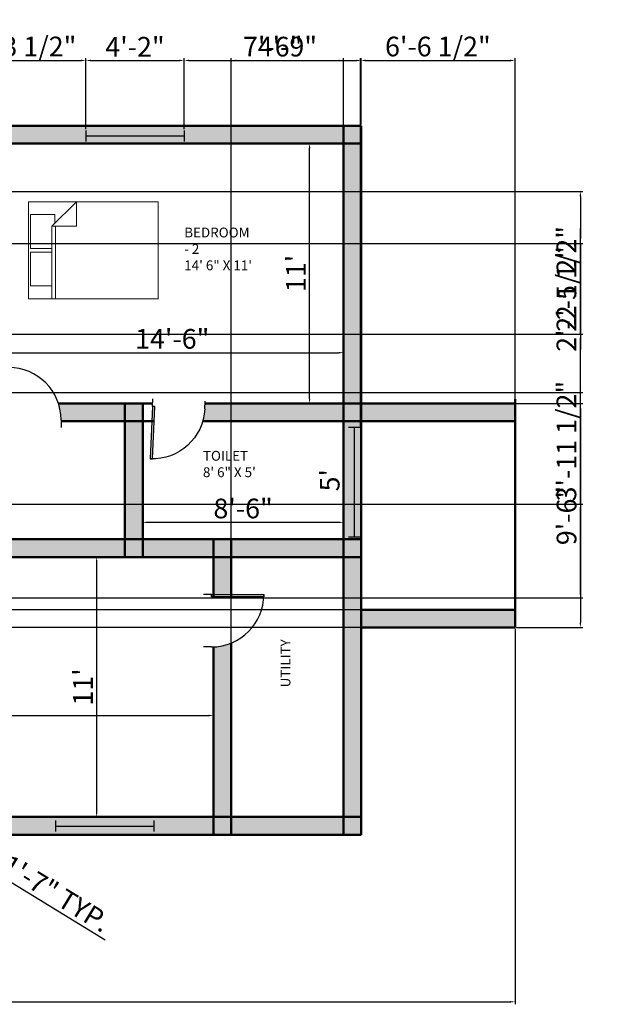
# Model space of a CAD drawing. Units: millimetres. Extents: x 2208 to 3043, y 878 to 1386.
# Tile 4 of 4: x 2749 to 3043, y 886 to 1386. Entities that reach past the tile are written whole.
import ezdxf

# ---------------------------------------------------------------- set-up
doc = ezdxf.new("R2010")
doc.units = ezdxf.units.MM
for name, color, linetype, lineweight in [('A-ANNO-DIMS', 50, 'Continuous', 13), ('A-AREA-IDEN', 90, 'Continuous', 25), ('A-WALL-PATT', 6, 'Continuous', 13), ('doors', 30, 'Continuous', 25), ('furniture', 140, 'Continuous', 18), ('walls', 200, 'Continuous', 50), ('windows', 10, 'Continuous', 25)]:
    doc.layers.add(name, color=color, linetype=linetype, lineweight=lineweight)
doc.styles.get("Standard").update_dxf_attribs({"font": 'arial.ttf'})
doc.dimstyles.new('ISO-25', dxfattribs={"dimtxt": 10, "dimasz": 2.5, "dimexe": 1.25, "dimexo": 0.625, "dimtad": 1, "dimdec": 0, "dimlunit": 3, "dimtxsty": 'Standard', "dimcen": 2.5, "dimadec": 0, "dimazin": 0, "dimtfac": 1, "dimtdec": 0, "dimtmove": 0, "dimatfit": 3, "dimfxl": 1, "dimarcsym": 0})

# ---------------------------------------------------------------- blocks, each defined once
blk = doc.blocks.new('*U2')
for p, q in [((0, 0), (0, -6)), ((40, 0), (40, -6))]:
    blk.add_line(p, q)
blk.add_lwpolyline([(0, 0), (0, 40), (1.75, 40), (1.75, 0)], close=True)
blk.add_arc((0, 0), 40, 0, 90)
blk = doc.blocks.new('*U4')
for p, q in [((0, 4), (0, 0)), ((36, 4), (36, 0)), ((0, 2), (36, 2))]:
    blk.add_line(p, q)
blk = doc.blocks.new('*U5')
for p, q in [((0, 4), (0, 0)), ((36, 4), (36, 0)), ((0, 2), (36, 2))]:
    blk.add_line(p, q)
blk = doc.blocks.new('Bed - Queen')
for p, q in [((0, -80.00003), (0, 0)), ((0, 0), (59.99999, 0)), ((59.99999, 0), (59.99999, -80.00003)), ((7.99999, -1.2), (28.79998, -1.2)), ((7.99999, -14.4), (7.99999, -1.2)), ((28.79998, -1.2), (28.79998, -14.4)), ((31.19999, -1.2), (51.99999, -1.2)), ((31.19999, -14.4), (31.19999, -1.2)), ((51.99999, -1.2), (51.99999, -16.4)), ((0, -14.4), (44.8, -14.4)), ((44.8, -16.8), (0, -16.8)), ((59.99999, -29.6), (44.8, -14.4)), ((44.8, -14.4), (44.8, -29.6)), ((51.99999, -16.4), (46.79936, -16.4)), ((44.8, -29.6), (59.99999, -29.6)), ((59.99999, -80.00003), (0, -80.00003))]:
    blk.add_line(p, q)
blk = doc.blocks.new('*D19')
at = {"layer": 'A-ANNO-DIMS', "color": 0, "lineweight": -2, "transparency": 16777216}
for p, q in [((2739.98, 1223.81), (2739.98, 1215.95)), ((2913.98, 1223.81), (2913.98, 1215.95)), ((2742.48, 1217.2), (2911.48, 1217.2))]:
    blk.add_line(p, q, dxfattribs=at)
at = {"layer": 'A-ANNO-DIMS', "color": 0, "transparency": 16777216}
for points in [[(2742.48, 1217.62), (2742.48, 1216.78), (2739.98, 1217.2)], [(2911.48, 1217.62), (2911.48, 1216.78), (2913.98, 1217.2)]]:
    blk.add_solid(points, dxfattribs=at)
at = {"layer": 'Defpoints', "color": 0, "transparency": 16777216}
for p in [(2739.98, 1224.44), (2913.98, 1224.44), (2913.98, 1217.2)]:
    blk.add_point(p, dxfattribs=at)
at = {"layer": 'A-ANNO-DIMS', "color": 0, "transparency": 16777216, "insert": (2826.98, 1222.93), "char_height": 10, "attachment_point": 5}
blk.add_mtext('14\'-6"', dxfattribs=at)
blk = doc.blocks.new('*D20')
at = {"layer": 'A-ANNO-DIMS', "color": 0, "lineweight": -2, "transparency": 16777216}
for p, q in [((2887.05, 1323.44), (2898, 1323.44)), ((2896.75, 1193.94), (2896.75, 1320.94)), ((2887.05, 1191.44), (2898, 1191.44))]:
    blk.add_line(p, q, dxfattribs=at)
at = {"layer": 'A-ANNO-DIMS', "color": 0, "transparency": 16777216}
for points in [[(2896.33, 1320.94), (2897.16, 1320.94), (2896.75, 1323.44)], [(2896.33, 1193.94), (2897.16, 1193.94), (2896.75, 1191.44)]]:
    blk.add_solid(points, dxfattribs=at)
at = {"layer": 'Defpoints', "color": 0, "transparency": 16777216}
for p in [(2886.43, 1323.44), (2896.75, 1323.44), (2886.43, 1191.44)]:
    blk.add_point(p, dxfattribs=at)
at = {"layer": 'A-ANNO-DIMS', "color": 0, "transparency": 16777216, "insert": (2891.1, 1257.44), "char_height": 10, "attachment_point": 5, "rotation": 90}
blk.add_mtext("11'", dxfattribs=at)
blk = doc.blocks.new('*D27')
at = {"layer": 'A-ANNO-DIMS', "color": 0, "lineweight": -2, "transparency": 16777216}
for p, q in [((2598.98, 1051.4), (2598.98, 1031.71)), ((2847.98, 1051.4), (2847.98, 1031.71)), ((2601.48, 1032.96), (2845.48, 1032.96))]:
    blk.add_line(p, q, dxfattribs=at)
at = {"layer": 'A-ANNO-DIMS', "color": 0, "transparency": 16777216}
for points in [[(2601.48, 1033.38), (2601.48, 1032.54), (2598.98, 1032.96)], [(2845.48, 1033.38), (2845.48, 1032.54), (2847.98, 1032.96)]]:
    blk.add_solid(points, dxfattribs=at)
at = {"layer": 'Defpoints', "color": 0, "transparency": 16777216}
for p in [(2598.98, 1052.02), (2847.98, 1052.02), (2847.98, 1032.96)]:
    blk.add_point(p, dxfattribs=at)
at = {"layer": 'A-ANNO-DIMS', "color": 0, "transparency": 16777216, "insert": (2723.48, 1038.69), "char_height": 10, "attachment_point": 5}
blk.add_mtext('20\'-9"', dxfattribs=at)
blk = doc.blocks.new('*D28')
at = {"layer": 'A-ANNO-DIMS', "color": 0, "lineweight": -2, "transparency": 16777216}
for p, q in [((2764.06, 1113.44), (2789.84, 1113.44)), ((2788.59, 1110.94), (2788.59, 983.94)), ((2764.06, 981.44), (2789.84, 981.44))]:
    blk.add_line(p, q, dxfattribs=at)
at = {"layer": 'A-ANNO-DIMS', "color": 0, "transparency": 16777216}
for points in [[(2788.18, 1110.94), (2789.01, 1110.94), (2788.59, 1113.44)], [(2788.18, 983.94), (2789.01, 983.94), (2788.59, 981.44)]]:
    blk.add_solid(points, dxfattribs=at)
at = {"layer": 'Defpoints', "color": 0, "transparency": 16777216}
for p in [(2763.44, 1113.44), (2763.44, 981.44), (2788.59, 981.44)]:
    blk.add_point(p, dxfattribs=at)
at = {"layer": 'A-ANNO-DIMS', "color": 0, "transparency": 16777216, "insert": (2782.95, 1047.44), "char_height": 10, "attachment_point": 5, "rotation": 90}
blk.add_mtext("11'", dxfattribs=at)
blk = doc.blocks.new('*D29')
at = {"layer": 'A-ANNO-DIMS', "color": 0, "lineweight": -2, "transparency": 16777216}
for p, q in [((2811.98, 1144.04), (2811.98, 1129.82)), ((2913.98, 1144.04), (2913.98, 1129.82)), ((2814.48, 1131.07), (2911.48, 1131.07))]:
    blk.add_line(p, q, dxfattribs=at)
at = {"layer": 'A-ANNO-DIMS', "color": 0, "transparency": 16777216}
for points in [[(2814.48, 1131.48), (2814.48, 1130.65), (2811.98, 1131.07)], [(2911.48, 1131.48), (2911.48, 1130.65), (2913.98, 1131.07)]]:
    blk.add_solid(points, dxfattribs=at)
at = {"layer": 'Defpoints', "color": 0, "transparency": 16777216}
for p in [(2811.98, 1144.67), (2913.98, 1144.67), (2913.98, 1131.07)]:
    blk.add_point(p, dxfattribs=at)
at = {"layer": 'A-ANNO-DIMS', "color": 0, "transparency": 16777216, "insert": (2862.98, 1136.8), "char_height": 10, "attachment_point": 5}
blk.add_mtext('8\'-6"', dxfattribs=at)
blk = doc.blocks.new('*D30')
at = {"layer": 'A-ANNO-DIMS', "color": 0, "lineweight": -2, "transparency": 16777216}
for p, q in [((2900.41, 1182.44), (2915.23, 1182.44)), ((2913.98, 1124.94), (2913.98, 1179.94)), ((2900.41, 1122.44), (2915.23, 1122.44))]:
    blk.add_line(p, q, dxfattribs=at)
at = {"layer": 'A-ANNO-DIMS', "color": 0, "transparency": 16777216}
for points in [[(2913.57, 1179.94), (2914.4, 1179.94), (2913.98, 1182.44)], [(2913.57, 1124.94), (2914.4, 1124.94), (2913.98, 1122.44)]]:
    blk.add_solid(points, dxfattribs=at)
at = {"layer": 'Defpoints', "color": 0, "transparency": 16777216}
for p in [(2899.78, 1182.44), (2913.98, 1182.44), (2899.78, 1122.44)]:
    blk.add_point(p, dxfattribs=at)
at = {"layer": 'A-ANNO-DIMS', "color": 0, "transparency": 16777216, "insert": (2908.27, 1152.44), "char_height": 10, "attachment_point": 5, "rotation": 90}
blk.add_mtext("5'", dxfattribs=at)
blk = doc.blocks.new('*D38')
at = {"layer": 'A-ANNO-DIMS', "color": 0, "lineweight": -2, "transparency": 16777216}
for p, q in [((2680.05, 985.52), (2681.86, 988.48)), ((2683.34, 986.11), (2695.25, 978.83)), ((2696.22, 975.63), (2698.03, 978.59)), ((2697.38, 977.52), (2792.87, 919.11))]:
    blk.add_line(p, q, dxfattribs=at)
at = {"layer": 'A-ANNO-DIMS', "color": 0, "transparency": 16777216}
for points in [[(2683.56, 986.47), (2683.13, 985.76), (2681.21, 987.42)], [(2695.47, 979.18), (2695.03, 978.47), (2697.38, 977.52)]]:
    blk.add_solid(points, dxfattribs=at)
at = {"layer": 'Defpoints', "color": 0, "transparency": 16777216}
for p in [(2679.73, 984.99), (2695.9, 975.1), (2697.38, 977.52)]:
    blk.add_point(p, dxfattribs=at)
at = {"layer": 'A-ANNO-DIMS', "color": 0, "transparency": 16777216, "insert": (2749.21, 952.61), "char_height": 10, "attachment_point": 5, "rotation": 328.5439}
blk.add_mtext('CHAIR 1\'-7" TYP.', dxfattribs=at)
blk = doc.blocks.new('*D46')
at = {"layer": 'A-ANNO-DIMS', "color": 0, "lineweight": -2, "transparency": 16777216}
for p, q in [((3001.16, 1077), (3001.16, 886.32)), ((2343.98, 972.81), (2343.98, 886.32)), ((2346.48, 887.57), (2998.66, 887.57))]:
    blk.add_line(p, q, dxfattribs=at)
at = {"layer": 'A-ANNO-DIMS', "color": 0, "transparency": 16777216}
for points in [[(2346.48, 887.99), (2346.48, 887.16), (2343.98, 887.57)], [(2998.66, 887.99), (2998.66, 887.16), (3001.16, 887.57)]]:
    blk.add_solid(points, dxfattribs=at)
at = {"layer": 'Defpoints', "color": 0, "transparency": 16777216}
for p in [(3001.16, 1077.62), (2343.98, 973.44), (3001.16, 887.57)]:
    blk.add_point(p, dxfattribs=at)
at = {"layer": 'A-ANNO-DIMS', "color": 0, "transparency": 16777216, "insert": (2672.57, 893.3), "char_height": 10, "attachment_point": 5}
blk.add_mtext('54\'-9"', dxfattribs=at)
blk = doc.blocks.new('*D48')
at = {"layer": 'A-ANNO-DIMS', "color": 0, "lineweight": -2, "transparency": 16777216}
for p, q in [((2922.7, 1179.95), (2922.7, 1366.84)), ((2925.2, 1365.59), (2998.66, 1365.59)), ((3001.16, 1192.06), (3001.16, 1366.84))]:
    blk.add_line(p, q, dxfattribs=at)
at = {"layer": 'A-ANNO-DIMS', "color": 0, "transparency": 16777216}
for points in [[(2925.2, 1366), (2925.2, 1365.17), (2922.7, 1365.59)], [(2998.66, 1366), (2998.66, 1365.17), (3001.16, 1365.59)]]:
    blk.add_solid(points, dxfattribs=at)
at = {"layer": 'Defpoints', "color": 0, "transparency": 16777216}
for p in [(3001.16, 1365.59), (3001.16, 1191.44), (2922.7, 1179.32)]:
    blk.add_point(p, dxfattribs=at)
at = {"layer": 'A-ANNO-DIMS', "color": 0, "transparency": 16777216, "insert": (2961.93, 1371.38), "char_height": 10, "attachment_point": 5}
blk.add_mtext('6\'-6 1/2"', dxfattribs=at)
blk = doc.blocks.new('*D49')
at = {"layer": 'A-ANNO-DIMS', "color": 0, "lineweight": -2, "transparency": 16777216}
for p, q in [((3001.79, 1191.44), (3035.56, 1191.44)), ((3034.31, 1188.94), (3034.31, 1080.12)), ((3001.79, 1077.62), (3035.56, 1077.62))]:
    blk.add_line(p, q, dxfattribs=at)
at = {"layer": 'A-ANNO-DIMS', "color": 0, "transparency": 16777216}
for points in [[(3033.9, 1188.94), (3034.73, 1188.94), (3034.31, 1191.44)], [(3033.9, 1080.12), (3034.73, 1080.12), (3034.31, 1077.62)]]:
    blk.add_solid(points, dxfattribs=at)
at = {"layer": 'Defpoints', "color": 0, "transparency": 16777216}
for p in [(3001.16, 1191.44), (3001.16, 1077.62), (3034.31, 1077.62)]:
    blk.add_point(p, dxfattribs=at)
at = {"layer": 'A-ANNO-DIMS', "color": 0, "transparency": 16777216, "insert": (3028.58, 1134.53), "char_height": 10, "attachment_point": 5, "rotation": 90}
blk.add_mtext('9\'-6"', dxfattribs=at)
blk = doc.blocks.new('*D50')
at = {"layer": 'A-ANNO-DIMS', "color": 0, "lineweight": -2, "transparency": 16777216}
for p, q in [((2856.98, 973.06), (2856.98, 1366.84)), ((2859.48, 1365.59), (2911.48, 1365.59)), ((2913.98, 973.06), (2913.98, 1366.84))]:
    blk.add_line(p, q, dxfattribs=at)
at = {"layer": 'A-ANNO-DIMS', "color": 0, "transparency": 16777216}
for points in [[(2859.48, 1366), (2859.48, 1365.17), (2856.98, 1365.59)], [(2911.48, 1366), (2911.48, 1365.17), (2913.98, 1365.59)]]:
    blk.add_solid(points, dxfattribs=at)
at = {"layer": 'Defpoints', "color": 0, "transparency": 16777216}
for p in [(2913.98, 1365.59), (2856.98, 972.44), (2913.98, 972.44)]:
    blk.add_point(p, dxfattribs=at)
at = {"layer": 'A-ANNO-DIMS', "color": 0, "transparency": 16777216, "insert": (2885.48, 1371.32), "char_height": 10, "attachment_point": 5}
blk.add_mtext('4\'-9"', dxfattribs=at)
blk = doc.blocks.new('*D51')
at = {"layer": 'A-ANNO-DIMS', "color": 0, "lineweight": -2, "transparency": 16777216}
for p, q in [((2344.15, 1299.03), (3035.56, 1299.03)), ((3034.31, 1296.53), (3034.31, 1275.14)), ((2344.61, 1272.64), (3035.56, 1272.64)), ((3034.31, 1272.64), (3034.31, 1218.83))]:
    blk.add_line(p, q, dxfattribs=at)
at = {"layer": 'A-ANNO-DIMS', "color": 0, "transparency": 16777216}
for points in [[(3033.9, 1296.53), (3034.73, 1296.53), (3034.31, 1299.03)], [(3033.9, 1275.14), (3034.73, 1275.14), (3034.31, 1272.64)]]:
    blk.add_solid(points, dxfattribs=at)
at = {"layer": 'Defpoints', "color": 0, "transparency": 16777216}
for p in [(2343.52, 1299.03), (2343.98, 1272.64), (3034.31, 1272.64)]:
    blk.add_point(p, dxfattribs=at)
at = {"layer": 'A-ANNO-DIMS', "color": 0, "transparency": 16777216, "insert": (3028.52, 1244.49), "char_height": 10, "attachment_point": 5, "rotation": 90}
blk.add_mtext('2\'-2 1/2"', dxfattribs=at)
blk = doc.blocks.new('*D59')
at = {"layer": 'A-ANNO-DIMS', "color": 0, "lineweight": -2, "transparency": 16777216}
for p, q in [((2719.8, 1331.57), (2719.8, 1366.84)), ((2722.3, 1365.59), (2780.58, 1365.59)), ((2783.08, 1330.66), (2783.08, 1366.84))]:
    blk.add_line(p, q, dxfattribs=at)
at = {"layer": 'A-ANNO-DIMS', "color": 0, "transparency": 16777216}
for points in [[(2722.3, 1366), (2722.3, 1365.17), (2719.8, 1365.59)], [(2780.58, 1366), (2780.58, 1365.17), (2783.08, 1365.59)]]:
    blk.add_solid(points, dxfattribs=at)
at = {"layer": 'Defpoints', "color": 0, "transparency": 16777216}
for p in [(2783.08, 1365.59), (2719.8, 1330.94), (2783.08, 1330.03)]:
    blk.add_point(p, dxfattribs=at)
at = {"layer": 'A-ANNO-DIMS', "color": 0, "transparency": 16777216, "insert": (2751.44, 1371.38), "char_height": 10, "attachment_point": 5}
blk.add_mtext('5\'-3 1/2"', dxfattribs=at)
blk = doc.blocks.new('*D60')
at = {"layer": 'A-ANNO-DIMS', "color": 0, "lineweight": -2, "transparency": 16777216}
for p, q in [((2783.08, 1330.66), (2783.08, 1366.84)), ((2785.58, 1365.59), (2830.53, 1365.59)), ((2833.03, 1330.66), (2833.03, 1366.84))]:
    blk.add_line(p, q, dxfattribs=at)
at = {"layer": 'A-ANNO-DIMS', "color": 0, "transparency": 16777216}
for points in [[(2785.58, 1366), (2785.58, 1365.17), (2783.08, 1365.59)], [(2830.53, 1366), (2830.53, 1365.17), (2833.03, 1365.59)]]:
    blk.add_solid(points, dxfattribs=at)
at = {"layer": 'Defpoints', "color": 0, "transparency": 16777216}
for p in [(2833.03, 1365.59), (2783.08, 1330.03), (2833.03, 1330.03)]:
    blk.add_point(p, dxfattribs=at)
at = {"layer": 'A-ANNO-DIMS', "color": 0, "transparency": 16777216, "insert": (2808.06, 1371.23), "char_height": 10, "attachment_point": 5}
blk.add_mtext('4\'-2"', dxfattribs=at)
blk = doc.blocks.new('*D61')
at = {"layer": 'A-ANNO-DIMS', "color": 0, "lineweight": -2, "transparency": 16777216}
for p, q in [((2833.03, 1330.66), (2833.03, 1366.84)), ((2835.53, 1365.59), (2920.48, 1365.59)), ((2922.98, 1333.06), (2922.98, 1366.84))]:
    blk.add_line(p, q, dxfattribs=at)
at = {"layer": 'A-ANNO-DIMS', "color": 0, "transparency": 16777216}
for points in [[(2835.53, 1366), (2835.53, 1365.17), (2833.03, 1365.59)], [(2920.48, 1366), (2920.48, 1365.17), (2922.98, 1365.59)]]:
    blk.add_solid(points, dxfattribs=at)
at = {"layer": 'Defpoints', "color": 0, "transparency": 16777216}
for p in [(2922.98, 1365.59), (2833.03, 1330.03), (2922.98, 1332.44)]:
    blk.add_point(p, dxfattribs=at)
at = {"layer": 'A-ANNO-DIMS', "color": 0, "transparency": 16777216, "insert": (2878, 1371.32), "char_height": 10, "attachment_point": 5}
blk.add_mtext('7\'-6"', dxfattribs=at)
blk = doc.blocks.new('*D62')
at = {"layer": 'A-ANNO-DIMS', "color": 0, "lineweight": -2, "transparency": 16777216}
for p, q in [((2310.37, 1086.62), (2310.37, 1116.95)), ((3000.54, 1086.62), (2309.12, 1086.62)), ((2310.37, 1080.12), (2310.37, 1084.12)), ((3000.54, 1077.62), (2309.12, 1077.62))]:
    blk.add_line(p, q, dxfattribs=at)
at = {"layer": 'A-ANNO-DIMS', "color": 0, "transparency": 16777216}
for points in [[(2309.95, 1084.12), (2310.79, 1084.12), (2310.37, 1086.62)], [(2309.95, 1080.12), (2310.79, 1080.12), (2310.37, 1077.62)]]:
    blk.add_solid(points, dxfattribs=at)
at = {"layer": 'Defpoints', "color": 0, "transparency": 16777216}
for p in [(2310.37, 1086.62), (3001.16, 1086.62), (3001.16, 1077.62)]:
    blk.add_point(p, dxfattribs=at)
at = {"layer": 'A-ANNO-DIMS', "color": 0, "transparency": 16777216, "insert": (2304.64, 1103.04), "char_height": 10, "attachment_point": 5, "rotation": 90}
blk.add_mtext('0\'-9"', dxfattribs=at)
blk = doc.blocks.new('*D64')
at = {"layer": 'A-ANNO-DIMS', "color": 0, "lineweight": -2, "transparency": 16777216}
for p, q in [((3034.31, 1226.55), (3034.31, 1280.35)), ((2465.97, 1226.55), (3035.56, 1226.55)), ((3034.31, 1199.41), (3034.31, 1224.05)), ((2465.97, 1196.91), (3035.56, 1196.91))]:
    blk.add_line(p, q, dxfattribs=at)
at = {"layer": 'A-ANNO-DIMS', "color": 0, "transparency": 16777216}
for points in [[(3033.9, 1224.05), (3034.73, 1224.05), (3034.31, 1226.55)], [(3033.9, 1199.41), (3034.73, 1199.41), (3034.31, 1196.91)]]:
    blk.add_solid(points, dxfattribs=at)
at = {"layer": 'Defpoints', "color": 0, "transparency": 16777216}
for p in [(2465.35, 1226.55), (3034.31, 1226.55), (2465.35, 1196.91)]:
    blk.add_point(p, dxfattribs=at)
at = {"layer": 'A-ANNO-DIMS', "color": 0, "transparency": 16777216, "insert": (3028.52, 1254.7), "char_height": 10, "attachment_point": 5, "rotation": 90}
blk.add_mtext('2\'-5 1/2"', dxfattribs=at)
blk = doc.blocks.new('*D66')
at = {"layer": 'A-ANNO-DIMS', "color": 0, "lineweight": -2, "transparency": 16777216}
for p, q in [((3034.31, 1140.35), (3034.31, 1201.74)), ((2674.33, 1140.35), (3035.56, 1140.35)), ((3034.31, 1095.26), (3034.31, 1137.85)), ((2673.86, 1092.76), (3035.56, 1092.76))]:
    blk.add_line(p, q, dxfattribs=at)
at = {"layer": 'A-ANNO-DIMS', "color": 0, "transparency": 16777216}
for points in [[(3033.9, 1137.85), (3034.73, 1137.85), (3034.31, 1140.35)], [(3033.9, 1095.26), (3034.73, 1095.26), (3034.31, 1092.76)]]:
    blk.add_solid(points, dxfattribs=at)
at = {"layer": 'Defpoints', "color": 0, "transparency": 16777216}
for p in [(2673.7, 1140.35), (3034.31, 1140.35), (2673.23, 1092.76)]:
    blk.add_point(p, dxfattribs=at)
at = {"layer": 'A-ANNO-DIMS', "color": 0, "transparency": 16777216, "insert": (3028.52, 1172.3), "char_height": 10, "attachment_point": 5, "rotation": 90}
blk.add_mtext('3\'-11 1/2"', dxfattribs=at)

msp = doc.modelspace()

# ---------------------------------------------------------------- hatches: boundary and pattern name
at = {"layer": 'A-WALL-PATT'}
h = msp.add_hatch(color=256, dxfattribs=at)
h.dxf.hatch_style = 1
h.paths.add_polyline_path([(2352.98, 1273, -0.051847), (2347.51, 1272.43), (2343.98, 1272.43), (2343.98, 1137.44), (2352.98, 1137.44)])
h.paths.add_polyline_path([(2352.98, 1323.44), (2343.98, 1323.44), (2343.98, 1299.03), (2347.51, 1299.03), (2352.98, 1299.03)])
h.paths.add_polyline_path([(2352.98, 1332.44), (2343.98, 1332.44), (2343.98, 1323.44), (2352.98, 1323.44)])
h.paths.add_polyline_path([(2496.98, 1332.44), (2352.98, 1332.44), (2352.98, 1323.44), (2496.98, 1323.44)])
h.paths.add_polyline_path([(2505.98, 1323.44), (2496.98, 1323.44), (2496.98, 1191.44), (2505.98, 1191.44)])
h.paths.add_polyline_path([(2505.98, 1332.44), (2496.98, 1332.44), (2496.98, 1323.44), (2505.98, 1323.44)])
h.paths.add_polyline_path([(2505.98, 1182.44), (2496.98, 1182.44), (2496.98, 1137.44), (2505.98, 1137.44)])
h.paths.add_polyline_path([(2505.98, 1191.44), (2496.98, 1191.44), (2496.98, 1182.44), (2505.98, 1182.44)])
h.paths.add_polyline_path([(2621.06, 1191.44), (2505.98, 1191.44), (2505.98, 1182.44), (2619.92, 1182.44), (2619.92, 1183.73, -0.073589)])
h.paths.add_polyline_path([(2496.98, 1137.44), (2352.98, 1137.44), (2352.98, 1128.44), (2496.98, 1128.44)])
h.paths.add_polyline_path([(2352.98, 1137.44), (2343.98, 1137.44), (2343.98, 1128.44), (2352.98, 1128.44)])
h.paths.add_polyline_path([(2352.98, 1128.44), (2343.98, 1128.44), (2343.98, 982.44), (2352.98, 982.44)])
h.paths.add_polyline_path([(2517.98, 1137.44), (2508.98, 1137.44), (2508.98, 1128.44), (2517.98, 1128.44)])
h.paths.add_polyline_path([(2505.98, 1137.44), (2496.98, 1137.44), (2496.98, 1128.44), (2505.98, 1128.44)])
h.paths.add_polyline_path([(2658.98, 1224.44), (2649.98, 1224.44), (2649.98, 1191.44), (2658.98, 1191.44)])
h.paths.add_polyline_path([(2658.98, 1323.44), (2649.98, 1323.44), (2649.98, 1233.44), (2658.98, 1233.44)])
h.paths.add_polyline_path([(2658.98, 1233.44), (2649.98, 1233.44), (2649.98, 1224.44), (2658.98, 1224.44)])
h.paths.add_polyline_path([(2730.98, 1233.44), (2658.98, 1233.44), (2658.98, 1224.44), (2730.98, 1224.44)])
h.paths.add_polyline_path([(2739.98, 1323.44), (2730.98, 1323.44), (2730.98, 1233.44), (2739.98, 1233.44)])
h.paths.add_polyline_path([(2739.98, 1224.44), (2730.98, 1224.44), (2730.98, 1191.44), (2739.98, 1191.44)])
h.paths.add_polyline_path([(2739.98, 1191.44), (2730.98, 1191.44), (2730.98, 1182.44), (2739.98, 1182.44)])
h.paths.add_polyline_path([(2739.98, 1182.44), (2730.98, 1182.44), (2730.98, 1171.44), (2739.98, 1171.44)])
h.paths.add_polyline_path([(2739.98, 972.44), (2730.98, 972.44), (2730.98, 929.72), (2602.15, 929.72), (2598.98, 929.72), (2598.98, 973.44), (2589.98, 973.44), (2589.98, 929.72), (2589.98, 920.72), (2730.98, 920.72), (2739.98, 920.72)])
h.paths.add_polyline_path([(2598.98, 1084.44), (2589.98, 1084.44), (2589.98, 982.44), (2598.98, 982.44)])
h.paths.add_polyline_path([(2598.98, 982.44), (2589.98, 982.44), (2589.98, 973.44), (2598.98, 973.44)])
h.paths.add_polyline_path([(2517.98, 973.44), (2508.98, 973.44), (2508.98, 944.53), (2517.98, 944.53)])
h.paths.add_polyline_path([(2517.98, 1044.76, -0.086498), (2508.98, 1043.19), (2508.98, 982.44), (2517.98, 982.44)])
h.paths.add_polyline_path([(2517.98, 982.44), (2508.98, 982.44), (2508.98, 973.44), (2517.98, 973.44)])
h.paths.add_polyline_path([(2352.98, 982.44), (2343.98, 982.44), (2343.98, 973.44), (2352.98, 973.44)])
h.paths.add_polyline_path([(2589.98, 1093.44), (2517.98, 1093.44), (2517.98, 1084.44), (2589.98, 1084.44)])
h.paths.add_polyline_path([(2517.98, 1093.44), (2508.98, 1093.44), (2508.98, 1084.44), (2517.98, 1084.44)])
h.paths.add_polyline_path([(2517.98, 1084.44), (2508.98, 1084.44), (2508.98, 1069.79), (2517.98, 1069.79)])
h.paths.add_polyline_path([(2517.98, 1100.83), (2517.21, 1100.83, -0.078775), (2508.98, 1102.14), (2508.98, 1093.44), (2517.98, 1093.44)])
h.paths.add_polyline_path([(2598.98, 1093.44), (2589.98, 1093.44), (2589.98, 1084.44), (2598.98, 1084.44)])
h.paths.add_polyline_path([(2802.98, 1122.44), (2730.98, 1122.44), (2730.98, 1113.44), (2802.98, 1113.44)])
h.paths.add_polyline_path([(2922.98, 1113.44), (2913.98, 1113.44), (2913.98, 981.44), (2922.98, 981.44)])
h.paths.add_polyline_path([(2856.98, 1069.77, -0.087206), (2847.98, 1067.81), (2847.98, 981.44), (2856.98, 981.44)])
h.paths.add_polyline_path([(2913.98, 981.44), (2856.98, 981.44), (2856.98, 972.44), (2913.98, 972.44)])
h.paths.add_polyline_path([(2856.98, 981.44), (2847.98, 981.44), (2847.98, 972.44), (2856.98, 972.44)])
h.paths.add_polyline_path([(2739.98, 995.72), (2739.98, 1004.72), (2730.98, 1004.72), (2730.98, 981.44), (2739.98, 981.44)])
h.paths.add_polyline_path([(2739.98, 981.44), (2730.98, 981.44), (2730.98, 972.44), (2739.98, 972.44)])
h.paths.add_polyline_path([(2922.98, 981.44), (2913.98, 981.44), (2913.98, 972.44), (2922.98, 972.44)])
h.paths.add_polyline_path([(3001.16, 1086.62), (2922.98, 1086.62), (2922.98, 1077.62), (3001.16, 1077.62)])
h.paths.add_polyline_path([(3001.16, 1191.44), (2922.98, 1191.44), (2922.98, 1182.44), (3001.16, 1182.44)])
h.paths.add_polyline_path([(2913.98, 1191.44), (2843.61, 1191.44), (2843.49, 1188.69, -0.05974), (2842.46, 1182.44), (2913.98, 1182.44)])
h.paths.add_polyline_path([(2922.98, 1191.44), (2913.98, 1191.44), (2913.98, 1182.44), (2922.98, 1182.44)])
h.paths.add_polyline_path([(2802.98, 1191.44), (2769.17, 1191.44, -0.079558), (2770.5, 1183.13), (2770.5, 1182.44), (2802.98, 1182.44)])
h.paths.add_polyline_path([(2811.98, 1191.44), (2802.98, 1191.44), (2802.98, 1182.44), (2811.98, 1182.44)])
h.paths.add_polyline_path([(2811.98, 1182.44), (2802.98, 1182.44), (2802.98, 1122.44), (2811.98, 1122.44)])
h.paths.add_polyline_path([(2811.98, 1122.44), (2802.98, 1122.44), (2802.98, 1113.44), (2811.98, 1113.44)])
h.paths.add_polyline_path([(2847.98, 1122.44), (2811.98, 1122.44), (2811.98, 1113.44), (2847.98, 1113.44)])
h.paths.add_polyline_path([(2856.98, 1122.44), (2847.98, 1122.44), (2847.98, 1113.44), (2856.98, 1113.44)])
h.paths.add_polyline_path([(2913.98, 1122.44), (2856.98, 1122.44), (2856.98, 1113.44), (2913.98, 1113.44)])
h.paths.add_polyline_path([(2922.98, 1122.44), (2913.98, 1122.44), (2913.98, 1113.44), (2922.98, 1113.44)])
h.paths.add_polyline_path([(2856.98, 1113.44), (2847.98, 1113.44), (2847.98, 1094.39), (2856.98, 1094.39)])
h.paths.add_polyline_path([(2922.98, 1323.44), (2913.98, 1323.44), (2913.98, 1191.44), (2922.98, 1191.44)])
h.paths.add_polyline_path([(2922.98, 1332.44), (2913.98, 1332.44), (2913.98, 1323.44), (2922.98, 1323.44)])
h.paths.add_polyline_path([(2913.98, 1332.44), (2739.98, 1332.44), (2739.98, 1323.44), (2913.98, 1323.44)])
h.paths.add_polyline_path([(2730.98, 1332.44), (2658.98, 1332.44), (2658.98, 1323.44), (2730.98, 1323.44)])
h.paths.add_polyline_path([(2649.98, 1332.44), (2505.98, 1332.44), (2505.98, 1323.44), (2649.98, 1323.44)])
h.paths.add_polyline_path([(2658.98, 1332.44), (2649.98, 1332.44), (2649.98, 1323.44), (2658.98, 1323.44)])
h.paths.add_polyline_path([(2739.98, 1332.44), (2730.98, 1332.44), (2730.98, 1323.44), (2739.98, 1323.44)])
h.paths.add_polyline_path([(2739.98, 1233.44), (2730.98, 1233.44), (2730.98, 1224.44), (2739.98, 1224.44)])
h.paths.add_polyline_path([(2658.98, 1191.44), (2649.98, 1191.44), (2649.98, 1182.44), (2658.98, 1182.44)])
h.paths.add_polyline_path([(2658.98, 1182.44), (2649.98, 1182.44), (2649.98, 1171.44), (2658.98, 1171.44)])
h.paths.add_polyline_path([(2508.98, 982.44), (2352.98, 982.44), (2352.98, 973.44), (2508.98, 973.44)])
h.paths.add_polyline_path([(2589.98, 982.44), (2517.98, 982.44), (2517.98, 973.44), (2589.98, 973.44)])
h.paths.add_polyline_path([(2730.98, 1004.72), (2598.98, 1004.72), (2598.98, 995.72), (2730.98, 995.72)])
h.paths.add_polyline_path([(2847.98, 981.44), (2739.98, 981.44), (2739.98, 972.44), (2847.98, 972.44)])
h = msp.add_hatch(color=256, dxfattribs=at)
h.dxf.hatch_style = 1
h.paths.add_polyline_path([(2922.98, 1182.44), (2913.98, 1182.44), (2913.98, 1122.44), (2922.98, 1122.44)])

# ---------------------------------------------------------------- linework, layer by layer
at = {"layer": 'walls'}
for p, q in [((2343.98, 1332.44), (2922.98, 1332.44)), ((2913.98, 1332.44), (2913.98, 972.44)), ((2922.98, 1332.44), (2922.98, 972.44)), ((2343.98, 1323.44), (2922.98, 1323.44)), ((2769.17, 1191.44), (2816.98, 1191.44)), ((2802.98, 1191.44), (2802.98, 1113.44)), ((2811.98, 1191.44), (2811.98, 1113.44)), ((2843.61, 1191.44), (3001.16, 1191.44)), ((3001.16, 1193.56), (3001.16, 1077.62)), ((2770.5, 1182.44), (2817.75, 1182.44)), ((2842.46, 1182.44), (3001.16, 1182.44)), ((2730.98, 1122.44), (2922.98, 1122.44)), ((2847.98, 1122.44), (2847.98, 1093.23)), ((2847.98, 1093.23), (2847.98, 1122.44)), ((2856.98, 1122.44), (2856.98, 1093.23)), ((2730.98, 1113.44), (2922.98, 1113.44)), ((2922.98, 1086.62), (3001.16, 1086.62)), ((2922.98, 1077.62), (3001.16, 1077.62)), ((2847.98, 1022.21), (2847.98, 1067.81)), ((2847.98, 1067.81), (2847.98, 972.44)), ((2856.98, 1069.77), (2856.98, 972.44)), ((2730.98, 981.44), (2922.98, 981.44)), ((2730.98, 972.44), (2922.98, 972.44))]:
    msp.add_line(p, q, dxfattribs=at)

# ---------------------------------------------------------------- block references
at = {"layer": 'doors', "xscale": 0.6650461219051067, "yscale": 0.6650461219051067, "zscale": 0.6650461219051067}
msp.add_blockref('*U2', (2743.9, 1183.13), dxfattribs=at)
at = {"layer": 'doors', "yscale": 0.6650461219051067, "zscale": 0.6650461219051067}
for p, xscale, rotation in [((2816.91, 1189.85), -0.6650461219051067, 177.4912975504383), ((2846.93, 1094.39), 0.6650461219051067, 270)]:
    msp.add_blockref('*U2', p, dxfattribs=dict(at, xscale=xscale, rotation=rotation))
at = {"layer": 'furniture', "xscale": 0.8230212393777605, "yscale": 0.8230212393777605, "zscale": 0.8230212393777605, "rotation": 90}
msp.add_blockref('Bed - Queen', (2753.92, 1244.5), dxfattribs=at)
at = {"layer": 'windows', "xscale": 1.38727767019332, "yscale": 1.38727767019332, "zscale": 1.38727767019332}
for p in [(2783.08, 1324.48), (2767.72, 974.08)]:
    msp.add_blockref('*U4', p, dxfattribs=at)
at = {"layer": 'windows', "xscale": 1.546623903893406, "yscale": 1.546623903893406, "zscale": 1.546623903893406, "rotation": 90}
msp.add_blockref('*U5', (2922.7, 1123.64), dxfattribs=at)

# ---------------------------------------------------------------- texts
at = {"layer": 'A-AREA-IDEN', "char_height": 5, "attachment_point": 1}
for s, width, insert in [('BEDROOM - 2\\P14\' 6" X 11\'', 34.627, (2833.07, 1280.73)), ('TOILET\\P8\' 6" X 5\'', 55.9776, (2842.57, 1167.34))]:
    msp.add_mtext_dynamic_manual_height_columns(s, width=width, gutter_width=12.5, heights=[0], dxfattribs=dict(at, insert=insert))
at = {"layer": 'A-AREA-IDEN', "insert": (2882.02, 1047.27), "char_height": 5, "attachment_point": 1, "rotation": 90}
msp.add_mtext_dynamic_manual_height_columns('UTILITY', width=51.8787, gutter_width=12.5, heights=[0], dxfattribs=at)

# ---------------------------------------------------------------- dimensions: what is measured, and where the dimension line sits
at = {"layer": 'A-ANNO-DIMS'}
for base, p1, p2, override, picture, middle in [((2783.08, 1365.59), (2719.8, 1330.94), (2783.08, 1330.03), {"dimdec": 1, "dimlfac": 1, "dimrnd": 0, "dimzin": 1, "dimdsep": 46, "dimlunit": 4, "dimfrac": 2}, '*D59', (2751.44, 1371.38)), ((3001.16, 1365.59), (2922.7, 1179.32), (3001.16, 1191.44), {"dimdec": 1, "dimlfac": 1, "dimrnd": 0, "dimzin": 1, "dimdsep": 46, "dimlunit": 4, "dimfrac": 2}, '*D48', (2961.93, 1371.38)), ((2833.0269, 1365.5855), (2783.0849, 1330.033), (2833.0269, 1330.033), {"dimdec": 1, "dimlfac": 1, "dimrnd": 0, "dimzin": 1, "dimdsep": 46, "dimlunit": 4, "dimfrac": 2}, '*D60', (2808.0559, 1371.231)), ((2922.9829, 1365.5855), (2833.0269, 1330.033), (2922.9829, 1332.4355), {"dimdec": 1, "dimlfac": 1, "dimrnd": 0, "dimzin": 1, "dimdsep": 46, "dimlunit": 4, "dimfrac": 2}, '*D61', (2878.0049, 1371.3162)), ((2913.98, 1365.59), (2856.98, 972.44), (2913.98, 972.44), {"dimdec": 1, "dimlfac": 1, "dimrnd": 0, "dimzin": 1, "dimdsep": 46, "dimlunit": 4, "dimfrac": 2}, '*D50', (2885.48, 1371.32)), ((2913.98, 1217.2), (2739.98, 1224.44), (2913.98, 1224.44), {"dimclrd": 0, "dimclre": 0, "dimclrt": 0}, '*D19', (2826.98, 1222.93)), ((2913.98, 1131.07), (2811.98, 1144.67), (2913.98, 1144.67), {"dimclrd": 0, "dimclre": 0, "dimclrt": 0}, '*D29', (2862.98, 1136.8)), ((3001.16, 887.57), (2343.98, 973.44), (3001.16, 1077.62), {"dimdec": 1, "dimlfac": 1, "dimrnd": 0, "dimzin": 1, "dimdsep": 46, "dimlunit": 4, "dimfrac": 2}, '*D46', (2672.57, 893.3)), ((2847.98, 1032.96), (2598.98, 1052.02), (2847.98, 1052.02), {"dimclrd": 0, "dimclre": 0, "dimclrt": 0}, '*D27', (2723.48, 1038.69))]:
    dim = msp.add_linear_dim(base=base, p1=p1, p2=p2, dimstyle='ISO-25', override=override, dxfattribs=at)
    dim.commit()
    dim.dimension.update_dxf_attribs({"geometry": picture, "text_midpoint": middle})
for base, p1, p2, override, picture, middle in [((2896.75, 1323.44), (2886.43, 1191.44), (2886.43, 1323.44), {"dimclrd": 0, "dimclre": 0, "dimclrt": 0}, '*D20', (2891.1, 1257.44)), ((3034.31, 1272.64), (2343.52, 1299.03), (2343.98, 1272.64), {"dimdec": 1, "dimlfac": 1, "dimrnd": 0, "dimzin": 1, "dimdsep": 46, "dimlunit": 4, "dimfrac": 2}, '*D51', (3028.52, 1244.49)), ((3034.31, 1226.55), (2465.35, 1196.91), (2465.35, 1226.55), {"dimdec": 1, "dimlfac": 1, "dimrnd": 0, "dimzin": 1, "dimdsep": 46, "dimlunit": 4, "dimfrac": 2}, '*D64', (3028.52, 1254.7)), ((3034.31, 1140.35), (2673.23, 1092.76), (2673.7, 1140.35), {"dimdec": 1, "dimlfac": 1, "dimrnd": 0, "dimzin": 1, "dimdsep": 46, "dimlunit": 4, "dimfrac": 2}, '*D66', (3028.52, 1172.3)), ((3034.31, 1077.62), (3001.16, 1191.44), (3001.16, 1077.62), {"dimdec": 1, "dimlfac": 1, "dimrnd": 0, "dimzin": 1, "dimdsep": 46, "dimlunit": 4, "dimfrac": 2}, '*D49', (3028.58, 1134.53)), ((2913.98, 1182.44), (2899.78, 1122.44), (2899.78, 1182.44), {"dimclrd": 0, "dimclre": 0, "dimclrt": 0}, '*D30', (2908.27, 1152.44)), ((2310.37, 1086.62), (3001.16, 1077.62), (3001.16, 1086.62), {"dimdec": 1, "dimlfac": 1, "dimrnd": 0, "dimzin": 1, "dimdsep": 46, "dimlunit": 4, "dimfrac": 2}, '*D62', (2304.64, 1103.04)), ((2788.59, 981.44), (2763.44, 1113.44), (2763.44, 981.44), {"dimclrd": 0, "dimclre": 0, "dimclrt": 0}, '*D28', (2782.95, 1047.44))]:
    dim = msp.add_linear_dim(base=base, p1=p1, p2=p2, angle=90, dimstyle='ISO-25', override=override, dxfattribs=at)
    dim.commit()
    dim.dimension.update_dxf_attribs({"geometry": picture, "text_midpoint": middle})
dim = msp.add_linear_dim(base=(2697.38, 977.52), p1=(2679.73, 984.99), p2=(2695.9, 975.1), angle=328.5439, text='CHAIR <> TYP.', dimstyle='ISO-25', override={"dimdec": 1, "dimlfac": 1, "dimrnd": 0, "dimzin": 1, "dimdsep": 46, "dimlunit": 4, "dimfrac": 2}, dxfattribs=at)
dim.commit()
dim.dimension.update_dxf_attribs({"geometry": '*D38', "text_midpoint": (2749.21, 952.61)})

doc.saveas('drawing.dxf')
